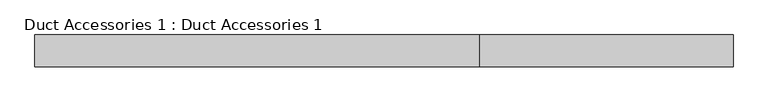
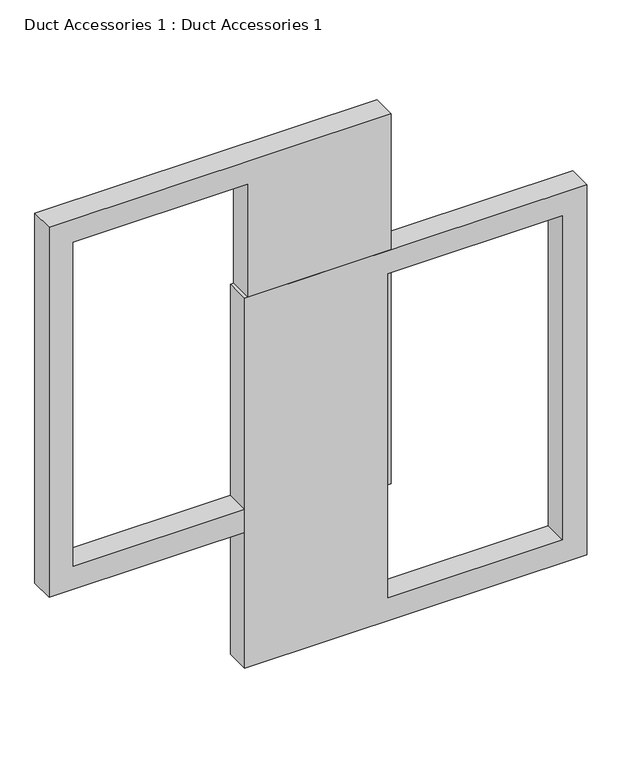
"""IFC4 building model written with IfcOpenShell, lengths in millimetres: damper geometry, Duct Accessories 1 : Duct Accessories 1."""

from ifc_helpers import new_model, si_unit, frame, origin, place, context, project, spatial, polyline, outline, extrude, source, transform, mapped, element, save


def duct_accessories_1_duct_accessories_1_838246fd(model_context):
    return source(origin(), model_context, "Body", "SweptSolid", [
        extrude(outline(polyline([(38222.7403114, -12928.36893), (37003.5403114, -12928.36893), (37003.5403114, -11861.56893), (38222.7403114, -11861.56893), (38222.7403114, -12928.36893)]), holes=[polyline([(38146.5403114, -12480.9324751), (38146.5403114, -11937.76893), (37079.7403114, -11937.76893), (37079.7403114, -12480.9324751), (38146.5403114, -12480.9324751)])]), frame((0.0, -447.4934478, 0.0), z_axis=(0.0, 1.0, 0.0), x_axis=(0.0, 0.0, 1.0)), (0.0, 0.0, 1.0), 76.2),
        extrude(outline(polyline([(38670.1767663, -12471.5606701), (38670.1767663, -13538.3606701), (37450.9767663, -13538.3606701), (37450.9767663, -12471.5606701), (38670.1767663, -12471.5606701)]), holes=[polyline([(38593.9767663, -12918.997125), (37527.1767663, -12918.997125), (37527.1767663, -13462.1606701), (38593.9767663, -13462.1606701), (38593.9767663, -12918.997125)])]), frame((0.0, -447.4934478, 0.0), z_axis=(0.0, 1.0, 0.0), x_axis=(0.0, 0.0, 1.0)), (0.0, 0.0, 1.0), 76.2),
    ])


if __name__ == "__main__":
    model = new_model("IFC4")
    model_context = context("Model", 3, world=origin())
    ifc_project = project(units=[si_unit("LENGTHUNIT", "METRE", prefix="MILLI")], contexts=[model_context])
    site = spatial("IfcSite", under=ifc_project)
    building = spatial("IfcBuilding", under=site)
    placement = place(None, origin())
    duct_accessories_1_duct_accessories_1_shape = duct_accessories_1_duct_accessories_1_838246fd(model_context)
    element("IfcDamper", 1, ObjectType="Duct Accessories 1 : Duct Accessories 1", at=placement, inside=building, context=model_context, shape_type="MappedRepresentation", body=[
        mapped(duct_accessories_1_duct_accessories_1_shape, transform((0.0, 0.0, 0.0), x_axis=(1.0, 0.0, 0.0), y_axis=(0.0, 1.0, 0.0), z_axis=(0.0, 0.0, 1.0))),
    ])
    save(model, "model.ifc")

# Revit data of these elements
# Element 1 (IfcDamper, "Duct Accessories 1 : Duct Accessories 1")
#   Materials on its faces: "border"
# Materials
#   "border": class "Generic", colour RGB 144 144 144, transparency 0, Cost = 0
